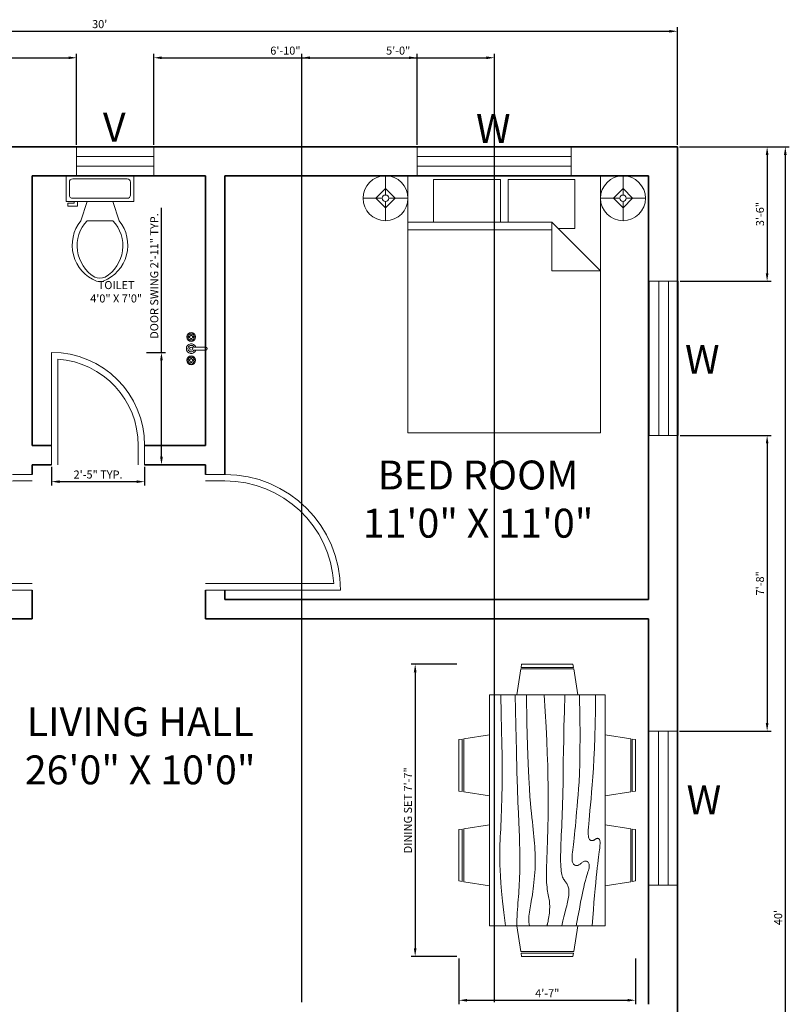
# Model space of a CAD drawing. Units: inches. Extents: x 1025 to 3479, y 1594 to 2212.
# Tile 3 of 9: x 1954 to 2194, y 1843 to 2150. Entities that reach past the tile are written whole.
import ezdxf

# ---------------------------------------------------------------- set-up
doc = ezdxf.new("R2010")
doc.units = ezdxf.units.IN
for name, color, linetype, lineweight in [('A-ANNO-DIMS', 1, 'Continuous', 18), ('A-ANNO-TEXT', 7, 'Continuous', 18), ('A-AREA-IDEN', 4, 'Continuous', 18), ('A-DOOR', 4, 'Continuous', 18), ('A-FLOR-FIXT', 9, 'Continuous', 18), ('A-FURN', 8, 'Continuous', 13), ('A-GLAZ', 3, 'Continuous', 18), ('A-WALL', 7, 'Continuous', 35)]:
    doc.layers.add(name, color=color, linetype=linetype, lineweight=lineweight)
doc.styles.get("Standard").update_dxf_attribs({"font": 'arial.ttf'})
doc.dimstyles.new('ISO-25', dxfattribs={"dimtxt": 2.5, "dimasz": 2.5, "dimexe": 1.25, "dimexo": 0.625, "dimtad": 1, "dimdec": 0, "dimlunit": 3, "dimtxsty": 'Standard', "dimcen": 2.5, "dimadec": 0, "dimazin": 0, "dimtfac": 1, "dimtdec": 0, "dimtmove": 0, "dimatfit": 3, "dimfxl": 1, "dimarcsym": 0})

# ---------------------------------------------------------------- blocks, each defined once
blk = doc.blocks.new('*D1')
at = {"layer": 'A-ANNO-DIMS', "color": 0, "lineweight": -2, "transparency": 16777216}
for p, q in [((1799.1, 2111.11), (1799.1, 2147.74)), ((1801.6, 2146.49), (2156.6, 2146.49)), ((2159.1, 2111.11), (2159.1, 2147.74))]:
    blk.add_line(p, q, dxfattribs=at)
at = {"layer": 'A-ANNO-DIMS', "color": 0, "transparency": 16777216}
for points in [[(1801.6, 2146.9), (1801.6, 2146.07), (1799.1, 2146.49)], [(2156.6, 2146.9), (2156.6, 2146.07), (2159.1, 2146.49)]]:
    blk.add_solid(points, dxfattribs=at)
at = {"layer": 'Defpoints', "color": 0, "transparency": 16777216}
for p in [(2159.1, 2146.49), (1799.1, 2110.49), (2159.1, 2110.49)]:
    blk.add_point(p, dxfattribs=at)
at = {"layer": 'A-ANNO-DIMS', "color": 0, "transparency": 16777216, "insert": (1979.1, 2148.39), "char_height": 2.5, "attachment_point": 5}
blk.add_mtext("30'", dxfattribs=at)
blk = doc.blocks.new('*D4')
at = {"layer": 'A-ANNO-DIMS', "color": 0, "lineweight": -2, "transparency": 16777216}
for p, q in [((2159.72, 2110.49), (2193.95, 2110.49)), ((2192.7, 2107.99), (2192.7, 1632.99)), ((2159.72, 1630.49), (2193.95, 1630.49))]:
    blk.add_line(p, q, dxfattribs=at)
at = {"layer": 'A-ANNO-DIMS', "color": 0, "transparency": 16777216}
for points in [[(2192.28, 2107.99), (2193.12, 2107.99), (2192.7, 2110.49)], [(2192.28, 1632.99), (2193.12, 1632.99), (2192.7, 1630.49)]]:
    blk.add_solid(points, dxfattribs=at)
at = {"layer": 'Defpoints', "color": 0, "transparency": 16777216}
for p in [(2159.1, 2110.49), (2159.1, 1630.49), (2192.7, 1630.49)]:
    blk.add_point(p, dxfattribs=at)
at = {"layer": 'A-ANNO-DIMS', "color": 0, "transparency": 16777216, "insert": (2190.8, 1870.49), "char_height": 2.5, "attachment_point": 5, "rotation": 90}
blk.add_mtext("40'", dxfattribs=at)
blk = doc.blocks.new('Dining Set - 36 x 72 in.')
for p, q in [((-22.2343, 26.00059), (-23.4847, 17.99762)), ((-22.2304, 26), (-5.7608, 26)), ((-22, 27.5), (-22.1562, 26.50042)), ((-5.8416, 26.5), (-22.1534, 26.5)), ((-22, 27.5), (-6, 27.5)), ((-5.8437, 26.49966), (-6, 27.5)), ((-4.5152, 17.99762), (-5.7655, 25.99926)), ((5.7657, 26.00059), (4.5153, 17.99762)), ((5.7696, 26), (22.2392, 26)), ((6, 27.5), (5.8438, 26.50042)), ((22.1584, 26.5), (5.8466, 26.5)), ((6, 27.5), (22, 27.5)), ((22.1563, 26.49966), (22, 27.5)), ((23.4848, 17.99762), (22.2345, 25.99926)), ((36, 18), (-36, 18)), ((-36, 18), (-36, -18)), ((36, -18), (36, 18)), ((-44.0006, 8.23428), (-35.9976, 9.48474)), ((44.0006, 8.23428), (35.9976, 9.48474)), ((-45.5, 8), (-44.5004, 8.15617)), ((-45.5, 8), (-45.5, -8)), ((-44.5, -8.15843), (-44.5, 8.15338)), ((-44, 8.23041), (-44, -8.23915)), ((44, 8.23041), (44, -8.23915)), ((44.5, -8.15843), (44.5, 8.15338)), ((45.5, 8), (44.5005, 8.15617)), ((45.5, 8), (45.5, -8)), ((-44.4997, -8.15631), (-45.5, -8)), ((-35.9976, -9.48476), (-43.9993, -8.2345)), ((35.9976, -9.48476), (43.9993, -8.2345)), ((44.4997, -8.15631), (45.5, -8)), ((-36, -18), (36, -18)), ((-22.2343, -26.0006), (-23.4847, -17.99762)), ((-4.5152, -17.99762), (-5.7655, -25.99928)), ((5.7657, -26.0006), (4.5153, -17.99762)), ((23.4848, -17.99762), (22.2345, -25.99928)), ((-22.2304, -26), (-5.7608, -26)), ((-22, -27.5), (-22.1562, -26.50044)), ((-5.8416, -26.5), (-22.1534, -26.5)), ((-22, -27.5), (-6, -27.5)), ((-5.8437, -26.49967), (-6, -27.5)), ((5.7696, -26), (22.2392, -26)), ((6, -27.5), (5.8438, -26.50044)), ((22.1584, -26.5), (5.8466, -26.5)), ((6, -27.5), (22, -27.5)), ((22.1563, -26.49967), (22, -27.5))]:
    blk.add_line(p, q)
for points in [[(-36, 15), (-31.1772, 14.97754), (-26.8079, 14.91406), (-22.8538, 14.81543), (-19.276, 14.6875), (-16.0362, 14.53613), (-13.0957, 14.36718), (-10.4159, 14.18652), (-7.9583, 14), (-5.6904, 13.81315), (-3.6035, 13.63021), (-1.6954, 13.45508), (0.0365, 13.29166), (1.5945, 13.14388), (2.9811, 13.01562), (4.1988, 12.9108), (5.25, 12.83333), (6.1393, 12.78613), (6.8802, 12.76823), (7.4883, 12.77767), (7.9792, 12.8125), (8.3685, 12.87077), (8.6719, 12.95052), (8.9049, 13.0498), (9.0833, 13.16666), (9.2205, 13.29899), (9.3216, 13.44401), (9.3895, 13.59879), (9.4271, 13.76041), (9.4373, 13.92594), (9.4232, 14.09245), (9.3875, 14.257), (9.3333, 14.41666), (9.2638, 14.56917), (9.1836, 14.71484), (9.0975, 14.85465), (9.0104, 14.98958), (8.9272, 15.1206), (8.8529, 15.2487), (8.7922, 15.37483), (8.75, 15.5), (8.7305, 15.62467), (8.7344, 15.74739), (8.7617, 15.86621), (8.8125, 15.97916), (8.8867, 16.08431), (8.9844, 16.17968), (9.1055, 16.26334), (9.25, 16.33333), (9.4189, 16.38802), (9.6172, 16.42708), (9.8506, 16.45052), (10.125, 16.45833), (10.4463, 16.45052), (10.8203, 16.42708), (11.2529, 16.38802), (11.75, 16.33333), (12.3184, 16.26318), (12.9694, 16.17838), (13.7151, 16.07991), (14.5677, 15.96875), (15.5395, 15.84586), (16.6426, 15.71224), (17.8893, 15.56884), (19.2917, 15.41666), (20.859, 15.25667), (22.5879, 15.08984), (24.4721, 14.91715), (26.5052, 14.73958), (28.6809, 14.5581), (30.9929, 14.3737), (33.4347, 14.18733), (36, 14)], [(-36, 10), (-28.9766, 10.14274), (-23.1725, 10.20442), (-18.4241, 10.19775), (-14.5677, 10.13541), (-11.4399, 10.03011), (-8.877, 9.89453), (-6.7154, 9.74137), (-4.7917, 9.58333), (-2.9698, 9.43082), (-1.2246, 9.28515), (0.4415, 9.14534), (2.026, 9.01041), (3.5266, 8.87939), (4.9408, 8.7513), (6.266, 8.62516), (7.5, 8.5), (8.6411, 8.37549), (9.6914, 8.2539), (10.6538, 8.13818), (11.5312, 8.03125), (12.3267, 7.93603), (13.043, 7.85547), (13.6831, 7.79248), (14.25, 7.75), (14.7471, 7.7303), (15.1797, 7.73307), (15.5537, 7.75732), (15.875, 7.80208), (16.1494, 7.86637), (16.3828, 7.94922), (16.5811, 8.04964), (16.75, 8.16666), (16.8944, 8.29915), (17.0143, 8.44531), (17.1089, 8.60319), (17.1771, 8.77083), (17.218, 8.94629), (17.2305, 9.1276), (17.2137, 9.31282), (17.1667, 9.5), (17.0895, 9.6875), (16.987, 9.875), (16.8649, 10.0625), (16.7292, 10.25), (16.5856, 10.4375), (16.4401, 10.625), (16.2985, 10.8125), (16.1667, 11), (16.05, 11.18733), (15.9518, 11.3737), (15.8752, 11.5581), (15.8229, 11.73958), (15.798, 11.91715), (15.8034, 12.08984), (15.842, 12.25667), (15.9167, 12.41666), (16.0295, 12.56836), (16.1784, 12.70833), (16.3605, 12.83268), (16.5729, 12.9375), (16.8127, 13.01888), (17.0768, 13.07291), (17.3625, 13.0957), (17.6667, 13.08333), (17.9894, 13.03312), (18.3418, 12.94726), (18.7382, 12.82918), (19.1927, 12.68229), (19.7195, 12.51001), (20.3327, 12.31575), (21.0465, 12.10294), (21.875, 11.875), (22.8357, 11.63354), (23.959, 11.37304), (25.2786, 11.08618), (26.8282, 10.76562), (28.6414, 10.40405), (30.752, 9.99414), (33.1936, 9.52856), (36, 9)], [(-36, 5.5), (-30.7157, 5.3348), (-26.069, 5.20963), (-21.9946, 5.11767), (-18.4271, 5.05208), (-15.3009, 5.00602), (-12.5508, 4.97265), (-10.1112, 4.94515), (-7.9167, 4.91666), (-5.909, 4.88167), (-4.0586, 4.83984), (-2.3429, 4.79215), (-0.7396, 4.73958), (0.7739, 4.6831), (2.22, 4.6237), (3.6213, 4.56233), (5, 4.5), (6.373, 4.43782), (7.7344, 4.3776), (9.0723, 4.32129), (10.375, 4.27083), (11.6309, 4.22819), (12.8281, 4.19531), (13.9551, 4.17415), (15, 4.16666), (15.954, 4.17448), (16.819, 4.19791), (17.6001, 4.23698), (18.3021, 4.29166), (18.9299, 4.36198), (19.4883, 4.44791), (19.9823, 4.54948), (20.4167, 4.66666), (20.7969, 4.79899), (21.1302, 4.94401), (21.4245, 5.09879), (21.6875, 5.26041), (21.9271, 5.42594), (22.1511, 5.59245), (22.3672, 5.757), (22.5834, 5.91666), (22.8065, 6.06868), (23.0404, 6.21093), (23.2879, 6.34147), (23.5521, 6.45833), (23.8358, 6.55957), (24.142, 6.64323), (24.4735, 6.70735), (24.8334, 6.75), (25.2235, 6.76969), (25.642, 6.76692), (26.0858, 6.74267), (26.5521, 6.69791), (27.0379, 6.63362), (27.5404, 6.55078), (28.0565, 6.45036), (28.5834, 6.33333), (29.1242, 6.19987), (29.7071, 6.04687), (30.3661, 5.87044), (31.1354, 5.66666), (32.0493, 5.43164), (33.142, 5.16146), (34.4475, 4.85221), (36, 4.5)], [(-36, -1), (-30.7915, -0.6591), (-26.0195, -0.38216), (-21.6519, -0.16284), (-17.6563, 0.00521), (-14.0005, 0.12833), (-10.6523, 0.21289), (-7.5796, 0.26522), (-4.75, 0.29166), (-2.134, 0.29793), (0.2878, 0.28711), (2.5317, 0.26163), (4.6146, 0.22396), (6.5529, 0.17651), (8.3633, 0.12174), (10.0623, 0.06209), (11.6667, 0), (13.1899, -0.06201), (14.6341, -0.1211), (15.9982, -0.17432), (17.2813, -0.21875), (18.4823, -0.25147), (19.6003, -0.26953), (20.6343, -0.27002), (21.5834, -0.25), (22.4481, -0.20768), (23.2357, -0.14584), (23.9549, -0.06836), (24.6146, 0.02083), (25.2235, 0.11784), (25.7904, 0.21875), (26.3241, 0.31966), (26.8334, 0.41666), (27.3265, 0.50618), (27.8099, 0.58593), (28.2894, 0.65397), (28.7709, 0.70833), (29.2601, 0.74707), (29.763, 0.76823), (30.2855, 0.76985), (30.8334, 0.75), (31.4088, 0.70784), (31.9994, 0.64713), (32.589, 0.57275), (33.1615, 0.48958), (33.7008, 0.4025), (34.1908, 0.3164), (34.6153, 0.23616), (34.9584, 0.16666), (35.2099, 0.11165), (35.3848, 0.07031), (35.504, 0.04069), (35.5886, 0.02083), (35.6594, 0.00879), (35.7377, 0.0026), (35.8442, 0.00032), (36, 0)], [(-36, -6.5), (-27.1843, -6.31267), (-20.084, -6.1263), (-14.469, -5.9419), (-10.1094, -5.76042), (-6.7752, -5.58285), (-4.2363, -5.41016), (-2.2629, -5.24333), (-0.625, -5.08334), (0.8708, -4.93099), (2.2715, -4.78646), (3.5872, -4.64974), (4.8281, -4.52084), (6.0046, -4.39974), (7.127, -4.28646), (8.2053, -4.18099), (9.25, -4.08334), (10.2705, -3.99382), (11.2734, -3.91407), (12.2647, -3.84603), (13.25, -3.79167), (14.2354, -3.75293), (15.2266, -3.73177), (16.2295, -3.73015), (17.25, -3.75), (18.2912, -3.79248), (19.3451, -3.85547), (20.4009, -3.93604), (21.4479, -4.03125), (22.4754, -4.13819), (23.4727, -4.25391), (24.4289, -4.37549), (25.3334, -4.5), (26.1785, -4.62492), (26.9694, -4.74935), (27.7145, -4.87281), (28.4219, -4.99479), (29.1, -5.11483), (29.7572, -5.23242), (30.4016, -5.34709), (31.0417, -5.45834), (31.6837, -5.56437), (32.3262, -5.65821), (32.9658, -5.73153), (33.599, -5.77604), (34.2224, -5.78345), (34.8327, -5.74545), (35.4264, -5.65373), (36, -5.5)], [(-36, -10), (-26.4022, -9.81299), (-18.4675, -9.62891), (-11.9839, -9.45069), (-6.7396, -9.28125), (-2.5226, -9.12354), (0.8789, -8.98047), (3.6769, -8.85498), (6.0833, -8.75), (8.2767, -8.66765), (10.3021, -8.60677), (12.1712, -8.56543), (13.8958, -8.54167), (15.4876, -8.53353), (16.9583, -8.53907), (18.3197, -8.55632), (19.5834, -8.58334), (20.7616, -8.61841), (21.8685, -8.66081), (22.9188, -8.71004), (23.9271, -8.76563), (24.9081, -8.82707), (25.8763, -8.89388), (26.8465, -8.96558), (27.8334, -9.04167), (28.8474, -9.12118), (29.8828, -9.20117), (30.93, -9.27824), (31.9792, -9.34896), (33.0205, -9.40991), (34.0443, -9.45768), (35.0407, -9.48885), (36, -9.5)], [(-36, -14.5), (-30.0881, -14.33513), (-25.0332, -14.21224), (-20.7312, -14.12647), (-17.0781, -14.07292), (-13.97, -14.04671), (-11.3027, -14.04297), (-8.9724, -14.05681), (-6.875, -14.08334), (-4.9224, -14.11833), (-3.0905, -14.16016), (-1.3709, -14.20785), (0.2448, -14.26042), (1.7647, -14.3169), (3.1973, -14.3763), (4.5507, -14.43767), (5.8333, -14.5), (7.0554, -14.5621), (8.235, -14.62175), (9.3922, -14.67652), (10.5469, -14.72396), (11.7192, -14.76164), (12.929, -14.78711), (14.1965, -14.79794), (15.5417, -14.79167), (16.9933, -14.76424), (18.6152, -14.70508), (20.4804, -14.60197), (22.6615, -14.44271), (25.2312, -14.21509), (28.2624, -13.9069), (31.8277, -13.50594), (36, -13)]]:
    blk.add_lwpolyline(points)
blk = doc.blocks.new('Bed - Queen')
for p, q in [((0, -80.00003), (0, 0)), ((0, 0), (59.99999, 0)), ((59.99999, 0), (59.99999, -80.00003)), ((7.99999, -1.2), (28.79998, -1.2)), ((7.99999, -14.4), (7.99999, -1.2)), ((28.79998, -1.2), (28.79998, -14.4)), ((31.19999, -1.2), (51.99999, -1.2)), ((31.19999, -14.4), (31.19999, -1.2)), ((51.99999, -1.2), (51.99999, -16.4)), ((0, -14.4), (44.8, -14.4)), ((59.99999, -29.6), (44.8, -14.4)), ((44.8, -14.4), (44.8, -29.6)), ((44.8, -16.8), (0, -16.8)), ((51.99999, -16.4), (46.79936, -16.4)), ((44.8, -29.6), (59.99999, -29.6)), ((59.99999, -80.00003), (0, -80.00003))]:
    blk.add_line(p, q)
blk = doc.blocks.new('Lamp - Table')
for p, q in [((0, 7), (0, 1)), ((-1, 0), (-7, 0)), ((0, 3), (-3, 0)), ((-3, 0), (0, -3)), ((3, 0), (0, 3)), ((0, -3), (3, 0)), ((1, 0), (7, 0)), ((0, -1), (0, -7))]:
    blk.add_line(p, q)
for radius in [7, 1]:
    blk.add_circle((0, 0), radius)
blk = doc.blocks.new('Toilet - top')
for p, q in [((9.5, -6), (9.5, -2)), ((-10, -8.5), (-8, -8.5)), ((-10, -9.5), (-10, -8.5)), ((-8, -8.5), (-8, -8)), ((-7, -8), (-7, -9.5)), ((-4, -8), (-6, -14)), ((4, -8), (6, -14)), ((-7, -9.5), (-10, -9.5)), ((4, -14), (-4, -14))]:
    blk.add_line(p, q)
blk.add_lwpolyline([(10.5, -8), (10.5, 0), (-10.5, 0), (-10.5, -8)], close=True)
for points in [[(-9.5, -2), (-9.5, -6)], [(8.5, -1), (-8.5, -1)], [(-8.5, -7), (8.5, -7)]]:
    blk.add_lwpolyline(points)
for centre, radius, start, end in [((-8.62, -1.88), 0.884, 81.8699, 188.1301), ((8.62, -1.88), 0.884, 351.8699, 98.1301), ((-8.62, -6.12), 0.884, 171.8699, 278.1301), ((8.62, -6.12), 0.884, 261.8699, 8.1301), ((3.52, -21.58), 12.17, 141.4691, 247.9714), ((4.2, -21.82), 11.33, 136.3677, 238.9468), ((-3.52, -21.58), 12.17, 292.0284, 38.5307), ((-4.2, -21.82), 11.33, 301.053, 43.6321), ((0, -27.88), 4, 245.7318, 294.2682), ((0, -29), 4, 254.8605, 285.1395)]:
    blk.add_arc(centre, radius, start, end)
blk = doc.blocks.new('Faucet - Bathroom top')
for p, q in [((-4.107, 0.125), (-4.375, 0.125)), ((-3.75, 0.4788), (-3.75, 0.75)), ((-3.5, 0.482), (-3.5, 0.75)), ((-3.1461, 0.125), (-2.875, 0.125)), ((3.143, 0.125), (2.875, 0.125)), ((3.5, 0.4788), (3.5, 0.75)), ((3.75, 0.482), (3.75, 0.75)), ((4.1039, 0.125), (4.375, 0.125)), ((-4.1039, -0.125), (-4.375, -0.125)), ((-3.75, -0.4821), (-3.75, -0.75)), ((-3.5, -0.4789), (-3.5, -0.75)), ((-3.143, -0.125), (-2.875, -0.125)), ((-0.5, -0.8639), (-0.5, -4.5)), ((0.5, -4.5), (0.5, -0.8631)), ((3.1461, -0.125), (2.875, -0.125)), ((3.5, -0.4821), (3.5, -0.75)), ((3.75, -0.4789), (3.75, -0.75)), ((4.107, -0.125), (4.375, -0.125))]:
    blk.add_line(p, q)
for centre, radius in [((-3.625, 0), 1.375), ((-4.625, 0), 0.2795), ((-3.625, 0), 0.5), ((-3.625, 1), 0.2795), ((-2.625, 0), 0.2795), ((0, 0), 0.5), ((3.625, 0), 1.375), ((2.625, 0), 0.2795), ((3.625, 0), 0.5), ((3.625, 1), 0.2795), ((4.625, 0), 0.2795), ((-3.625, -1), 0.2795), ((3.625, -1), 0.2795)]:
    blk.add_circle(centre, radius)
for centre, radius, start, end in [((-3.625, 0), 1, 105.2407, 164.2093), ((-3.625, 0), 1, 16.44125, 74.07887), ((0, 0), 1.5, 289.6514, 250.3603), ((0, 0), 1, 300.3431, 239.7554), ((3.625, 0), 1, 106.12, 164.0884), ((3.625, 0), 1, 16.23422, 73.90469), ((-3.625, 0), 1, 196.2342, 253.9047), ((-3.625, 0), 1, 286.12, 344.0884), ((3.625, 0), 1, 196.4413, 254.0789), ((3.625, 0), 1, 285.2407, 344.2093), ((0, -4.5), 0.5, 180, 0)]:
    blk.add_arc(centre, radius, start, end)
blk = doc.blocks.new('WIN-48IN')
for p, q in [((0, 48), (0, 0)), ((9, 48), (0, 48)), ((3, 48), (3, 0)), ((6, 0), (6, 48)), ((9, 0), (9, 48)), ((0, 0), (9, 0))]:
    blk.add_line(p, q)
blk = doc.blocks.new('VENT-24IN')
for p, q in [((24, 9), (0, 9)), ((0, 9), (0, 0)), ((24, 0), (24, 9)), ((24, 6), (0, 6)), ((0, 3), (24, 3)), ((0, 0), (24, 0))]:
    blk.add_line(p, q)
blk = doc.blocks.new('DOOR-SWING-36IN')
for p, q in [((0, 36), (6, 36)), ((0, 34), (6, 34)), ((0, 2), (6, 2)), ((6, 0), (0, 0)), ((6, 2), (39.94, 2)), ((6, 0), (42, 0))]:
    blk.add_line(p, q)
for radius, start in [(36, 0), (34, 3.3723)]:
    blk.add_arc((6, 0), radius, start, 90)
blk = doc.blocks.new('DOOR-SWING-29IN')
for p, q in [((0, 6), (0, 35)), ((2, 6), (2, 32.93)), ((0, 6), (0, 0)), ((2, 6), (2, 0)), ((27, 0), (27, 6)), ((29, 0), (29, 6))]:
    blk.add_line(p, q)
for radius, end in [(29, 90), (27, 85.752)]:
    blk.add_arc((0, 6), radius, 0, end)
blk = doc.blocks.new('*D34')
at = {"layer": 'A-ANNO-DIMS', "color": 0, "lineweight": -2, "transparency": 16777216}
for p, q in [((1998.35, 2046.49), (1998.35, 2091.55)), ((1993.72, 2046.49), (1999.6, 2046.49)), ((1998.35, 2013.99), (1998.35, 2043.99)), ((1993.72, 2011.49), (1999.6, 2011.49))]:
    blk.add_line(p, q, dxfattribs=at)
at = {"layer": 'A-ANNO-DIMS', "color": 0, "transparency": 16777216}
for points in [[(1997.93, 2043.99), (1998.77, 2043.99), (1998.35, 2046.49)], [(1997.93, 2013.99), (1998.77, 2013.99), (1998.35, 2011.49)]]:
    blk.add_solid(points, dxfattribs=at)
at = {"layer": 'Defpoints', "color": 0, "transparency": 16777216}
for p in [(1993.1, 2046.49), (1998.35, 2046.49), (1993.1, 2011.49)]:
    blk.add_point(p, dxfattribs=at)
at = {"layer": 'A-ANNO-DIMS', "color": 0, "transparency": 16777216, "insert": (1996.43, 2070.27), "char_height": 2.5, "attachment_point": 5, "rotation": 90}
blk.add_mtext('DOOR SWING 2\'-11" TYP.', dxfattribs=at)
blk = doc.blocks.new('*D35')
at = {"layer": 'A-ANNO-DIMS', "color": 0, "lineweight": -2, "transparency": 16777216}
for p, q in [((1964.1, 2010.86), (1964.1, 2004.99)), ((1993.1, 2010.86), (1993.1, 2004.99)), ((1966.6, 2006.24), (1990.6, 2006.24))]:
    blk.add_line(p, q, dxfattribs=at)
at = {"layer": 'A-ANNO-DIMS', "color": 0, "transparency": 16777216}
for points in [[(1966.6, 2006.65), (1966.6, 2005.82), (1964.1, 2006.24)], [(1990.6, 2006.65), (1990.6, 2005.82), (1993.1, 2006.24)]]:
    blk.add_solid(points, dxfattribs=at)
at = {"layer": 'Defpoints', "color": 0, "transparency": 16777216}
for p in [(1964.1, 2011.49), (1993.1, 2011.49), (1993.1, 2006.24)]:
    blk.add_point(p, dxfattribs=at)
at = {"layer": 'A-ANNO-DIMS', "color": 0, "transparency": 16777216, "insert": (1978.6, 2008.14), "char_height": 2.5, "attachment_point": 5}
blk.add_mtext('2\'-5" TYP.', dxfattribs=at)
blk = doc.blocks.new('*D44')
at = {"layer": 'A-ANNO-DIMS', "color": 0, "lineweight": -2, "transparency": 16777216}
for p, q in [((2090.41, 1949.4), (2076.14, 1949.4)), ((2077.39, 1946.9), (2077.39, 1860.9)), ((2090.41, 1858.4), (2076.14, 1858.4))]:
    blk.add_line(p, q, dxfattribs=at)
at = {"layer": 'A-ANNO-DIMS', "color": 0, "transparency": 16777216}
for points in [[(2076.97, 1946.9), (2077.81, 1946.9), (2077.39, 1949.4)], [(2076.97, 1860.9), (2077.81, 1860.9), (2077.39, 1858.4)]]:
    blk.add_solid(points, dxfattribs=at)
at = {"layer": 'Defpoints', "color": 0, "transparency": 16777216}
for p in [(2091.04, 1949.4), (2077.39, 1858.4), (2091.04, 1858.4)]:
    blk.add_point(p, dxfattribs=at)
at = {"layer": 'A-ANNO-DIMS', "color": 0, "transparency": 16777216, "insert": (2075.47, 1903.9), "char_height": 2.5, "attachment_point": 5, "rotation": 90}
blk.add_mtext('DINING SET 7\'-7"', dxfattribs=at)
blk = doc.blocks.new('*D45')
at = {"layer": 'A-ANNO-DIMS', "color": 0, "lineweight": -2, "transparency": 16777216}
for p, q in [((2091.04, 1857.77), (2091.04, 1843.5)), ((2146.04, 1857.77), (2146.04, 1843.5)), ((2093.54, 1844.75), (2143.54, 1844.75))]:
    blk.add_line(p, q, dxfattribs=at)
at = {"layer": 'A-ANNO-DIMS', "color": 0, "transparency": 16777216}
for points in [[(2093.54, 1845.16), (2093.54, 1844.33), (2091.04, 1844.75)], [(2143.54, 1845.16), (2143.54, 1844.33), (2146.04, 1844.75)]]:
    blk.add_solid(points, dxfattribs=at)
at = {"layer": 'Defpoints', "color": 0, "transparency": 16777216}
for p in [(2091.04, 1858.4), (2146.04, 1858.4), (2146.04, 1844.75)]:
    blk.add_point(p, dxfattribs=at)
at = {"layer": 'A-ANNO-DIMS', "color": 0, "transparency": 16777216, "insert": (2118.54, 1846.62), "char_height": 2.5, "attachment_point": 5}
blk.add_mtext('4\'-7"', dxfattribs=at)
blk = doc.blocks.new('*D50')
at = {"layer": 'A-ANNO-DIMS', "color": 0, "lineweight": -2, "transparency": 16777216}
for p, q in [((1876.48, 2111.11), (1876.48, 2139.49)), ((1878.98, 2138.24), (1969.43, 2138.24)), ((1971.93, 2111.11), (1971.93, 2139.49))]:
    blk.add_line(p, q, dxfattribs=at)
at = {"layer": 'A-ANNO-DIMS', "color": 0, "transparency": 16777216}
for points in [[(1878.98, 2138.65), (1878.98, 2137.82), (1876.48, 2138.24)], [(1969.43, 2138.65), (1969.43, 2137.82), (1971.93, 2138.24)]]:
    blk.add_solid(points, dxfattribs=at)
at = {"layer": 'Defpoints', "color": 0, "transparency": 16777216}
for p in [(1971.93, 2138.24), (1876.48, 2110.49), (1971.93, 2110.49)]:
    blk.add_point(p, dxfattribs=at)
at = {"layer": 'A-ANNO-DIMS', "color": 0, "transparency": 16777216, "insert": (1924.21, 2140.15), "char_height": 2.5, "attachment_point": 5}
blk.add_mtext('7\'-11 1/2"', dxfattribs=at)
blk = doc.blocks.new('*D51')
at = {"layer": 'A-ANNO-DIMS', "color": 0, "lineweight": -2, "transparency": 16777216}
for p, q in [((1995.93, 2111.11), (1995.93, 2139.49)), ((1998.43, 2138.24), (2075.48, 2138.24)), ((2077.98, 2111.11), (2077.98, 2139.49))]:
    blk.add_line(p, q, dxfattribs=at)
at = {"layer": 'A-ANNO-DIMS', "color": 0, "transparency": 16777216}
for points in [[(1998.43, 2138.65), (1998.43, 2137.82), (1995.93, 2138.24)], [(2075.48, 2138.65), (2075.48, 2137.82), (2077.98, 2138.24)]]:
    blk.add_solid(points, dxfattribs=at)
at = {"layer": 'Defpoints', "color": 0, "transparency": 16777216}
for p in [(2077.98, 2138.24), (1995.93, 2110.49), (2077.98, 2110.49)]:
    blk.add_point(p, dxfattribs=at)
at = {"layer": 'A-ANNO-DIMS', "color": 0, "transparency": 16777216, "insert": (2036.96, 2140.14), "char_height": 2.5, "attachment_point": 5}
blk.add_mtext('6\'-10"', dxfattribs=at)
blk = doc.blocks.new('*D69')
at = {"layer": 'A-ANNO-DIMS', "color": 0, "lineweight": -2, "transparency": 16777216}
for p, q in [((2159.72, 2110.49), (2188.29, 2110.49)), ((2187.04, 2107.99), (2187.04, 2071.13)), ((2159.91, 2068.63), (2188.29, 2068.63))]:
    blk.add_line(p, q, dxfattribs=at)
at = {"layer": 'A-ANNO-DIMS', "color": 0, "transparency": 16777216}
for points in [[(2186.62, 2107.99), (2187.46, 2107.99), (2187.04, 2110.49)], [(2186.62, 2071.13), (2187.46, 2071.13), (2187.04, 2068.63)]]:
    blk.add_solid(points, dxfattribs=at)
at = {"layer": 'Defpoints', "color": 0, "transparency": 16777216}
for p in [(2159.1, 2110.49), (2159.29, 2068.63), (2187.04, 2068.63)]:
    blk.add_point(p, dxfattribs=at)
at = {"layer": 'A-ANNO-DIMS', "color": 0, "transparency": 16777216, "insert": (2185.14, 2089.56), "char_height": 2.5, "attachment_point": 5, "rotation": 90}
blk.add_mtext('3\'-6"', dxfattribs=at)
blk = doc.blocks.new('*D70')
at = {"layer": 'A-ANNO-DIMS', "color": 0, "lineweight": -2, "transparency": 16777216}
for p, q in [((2159.91, 2020.63), (2188.29, 2020.63)), ((2187.04, 2018.13), (2187.04, 1931.05)), ((2159.78, 1928.55), (2188.29, 1928.55))]:
    blk.add_line(p, q, dxfattribs=at)
at = {"layer": 'A-ANNO-DIMS', "color": 0, "transparency": 16777216}
for points in [[(2186.62, 2018.13), (2187.46, 2018.13), (2187.04, 2020.63)], [(2186.62, 1931.05), (2187.46, 1931.05), (2187.04, 1928.55)]]:
    blk.add_solid(points, dxfattribs=at)
at = {"layer": 'Defpoints', "color": 0, "transparency": 16777216}
for p in [(2159.29, 2020.63), (2159.16, 1928.55), (2187.04, 1928.55)]:
    blk.add_point(p, dxfattribs=at)
at = {"layer": 'A-ANNO-DIMS', "color": 0, "transparency": 16777216, "insert": (2185.14, 1974.59), "char_height": 2.5, "attachment_point": 5, "rotation": 90}
blk.add_mtext('7\'-8"', dxfattribs=at)
blk = doc.blocks.new('*D84')
at = {"layer": 'A-ANNO-DIMS', "color": 0, "lineweight": -2, "transparency": 16777216}
for p, q in [((2042.1, 1844.11), (2042.1, 2139.49)), ((2044.6, 2138.24), (2099.6, 2138.24)), ((2102.1, 1844.11), (2102.1, 2139.49))]:
    blk.add_line(p, q, dxfattribs=at)
at = {"layer": 'A-ANNO-DIMS', "color": 0, "transparency": 16777216}
for points in [[(2044.6, 2138.65), (2044.6, 2137.82), (2042.1, 2138.24)], [(2099.6, 2138.65), (2099.6, 2137.82), (2102.1, 2138.24)]]:
    blk.add_solid(points, dxfattribs=at)
at = {"layer": 'Defpoints', "color": 0, "transparency": 16777216}
for p in [(2102.1, 2138.24), (2042.1, 1843.49), (2102.1, 1843.49)]:
    blk.add_point(p, dxfattribs=at)
at = {"layer": 'A-ANNO-DIMS', "color": 0, "transparency": 16777216, "insert": (2072.1, 2140.14), "char_height": 2.5, "attachment_point": 5}
blk.add_mtext('5\'-0"', dxfattribs=at)

msp = doc.modelspace()

# ---------------------------------------------------------------- linework, layer by layer
at = {"layer": 'A-DOOR'}
for p, q in [((1958.1, 1972.49), (1952.1, 1972.49)), ((2012.1, 1972.49), (2018.1, 1972.49))]:
    msp.add_line(p, q, dxfattribs=at)
at = {"layer": 'A-WALL'}
for p, q in [((1799.1, 2110.49), (2159.1, 2110.49)), ((2159.1, 2110.49), (2159.1, 1630.49)), ((1958.1, 2101.49), (2012.1, 2101.49)), ((1958.1, 2017.49), (1958.1, 2101.49)), ((1958.1, 2017.49), (1958.1, 2101.49)), ((2012.1, 2101.49), (2012.1, 2017.49)), ((2018.1, 2101.49), (2018.1, 2008.49)), ((2018.1, 2101.49), (2150.1, 2101.49)), ((2150.1, 2101.49), (2150.1, 1969.49)), ((1958.1, 2017.49), (1964.1, 2017.49)), ((1958.1, 2017.49), (1964.1, 2017.49)), ((1993.1, 2017.49), (2012.1, 2017.49)), ((1958.1, 2011.49), (1964.1, 2011.49)), ((1958.1, 2011.49), (1958.1, 2011.49)), ((1958.1, 2011.49), (1958.1, 2008.49)), ((1958.1, 2008.49), (1958.1, 2011.49)), ((1958.1, 2008.49), (1958.1, 2011.49)), ((1993.1, 2011.49), (2012.1, 2011.49)), ((2012.1, 2011.49), (2012.1, 2008.49)), ((2012.1, 2011.49), (2012.1, 2008.49)), ((1958.1, 1963.49), (1958.1, 1972.49)), ((1958.1, 1963.49), (1958.1, 1972.49)), ((2012.1, 1972.49), (2012.1, 1963.49)), ((2018.1, 1972.49), (2018.1, 1969.49)), ((2018.1, 1969.49), (2150.1, 1969.49)), ((1808.1, 1963.49), (1958.1, 1963.49)), ((2012.1, 1963.49), (2150.1, 1963.49)), ((2150.1, 1963.49), (2150.1, 1843.49))]:
    msp.add_line(p, q, dxfattribs=at)

# ---------------------------------------------------------------- block references
at = {"layer": 'A-DOOR'}
for name, p in [('DOOR-SWING-29IN', (1964.1, 2011.49)), ('DOOR-SWING-36IN', (2012.1, 1972.49))]:
    msp.add_blockref(name, p, dxfattribs=at)
at = {"layer": 'A-DOOR', "extrusion": (0, 0, -1), "zscale": -1}
msp.add_blockref('DOOR-SWING-36IN', (-1958.1, 1972.49), dxfattribs=at)
at = {"layer": 'A-FLOR-FIXT'}
msp.add_blockref('Toilet - top', (1979.19, 2101.49), dxfattribs=at)
at = {"layer": 'A-FLOR-FIXT', "rotation": 90}
msp.add_blockref('Faucet - Bathroom top', (2007.6, 2047.66), dxfattribs=at)
at = {"layer": 'A-FURN'}
for name, p in [('Lamp - Table', (2068.14, 2094.49)), ('Bed - Queen', (2075.14, 2101.49)), ('Lamp - Table', (2142.14, 2094.49))]:
    msp.add_blockref(name, p, dxfattribs=at)
at = {"layer": 'A-FURN', "rotation": 270}
msp.add_blockref('Dining Set - 36 x 72 in.', (2118.54, 1903.9), dxfattribs=at)
at = {"layer": 'A-GLAZ'}
for name, p in [('VENT-24IN', (1971.93, 2101.49)), ('WIN-48IN', (2150.29, 2020.63)), ('WIN-48IN', (2150.16, 1880.55))]:
    msp.add_blockref(name, p, dxfattribs=at)
at = {"layer": 'A-GLAZ', "rotation": 269.9999999999989}
msp.add_blockref('WIN-48IN', (2077.98, 2110.49), dxfattribs=at)

# ---------------------------------------------------------------- texts
at = {"layer": 'A-ANNO-TEXT', "char_height": 9, "attachment_point": 1}
for s, width, insert in [('\\pxqc;{V}', 7.8272, (1979.73, 2121.13)), ('\\pxqc;W', 15.8719, (2093.79, 2120.73)), ('\\pxqc;W', 15.8719, (2158.9, 2048.84)), ('\\pxqc;W', 15.8719, (2159.41, 1911.64))]:
    msp.add_mtext_dynamic_manual_height_columns(s, width=width, gutter_width=12.5, heights=[0], dxfattribs=dict(at, insert=insert))
at = {"layer": 'A-AREA-IDEN', "attachment_point": 1}
for s, width, insert, char_height in [('\\pxqc;TOILET\\P4\'0" X 7\'0"', 47.6002, (1960.44, 2068.7), 2.5), ('\\pxqc;BED ROOM \\P11\'0" X 11\'0"', 93.2353, (2050.37, 2012.8), 9), ('\\pxqc;LIVING HALL\\P26\'0" X 10\'0"', 112.2145, (1935.6, 1935.99), 9)]:
    msp.add_mtext_dynamic_manual_height_columns(s, width=width, gutter_width=12.5, heights=[0], dxfattribs=dict(at, insert=insert, char_height=char_height))

# ---------------------------------------------------------------- dimensions: what is measured, and where the dimension line sits
at = {"layer": 'A-ANNO-DIMS'}
for base, p1, p2, override, picture, middle in [((2159.1, 2146.49), (1799.1, 2110.49), (2159.1, 2110.49), {"dimclrd": 0, "dimclre": 0, "dimclrt": 0}, '*D1', (1979.1, 2148.39)), ((1971.9348, 2138.2355), (1876.4813, 2110.4855), (1971.9348, 2110.4855), {"dimdec": 1, "dimlfac": 1, "dimrnd": 0, "dimzin": 1, "dimdsep": 46, "dimlunit": 4, "dimfrac": 2}, '*D50', (1924.208, 2140.1532)), ((2077.9791, 2138.2355), (1995.9348, 2110.4855), (2077.9791, 2110.4855), {"dimdec": 1, "dimlfac": 1, "dimrnd": 0, "dimzin": 1, "dimdsep": 46, "dimlunit": 4, "dimfrac": 2}, '*D51', (2036.9569, 2140.137)), ((2102.1, 2138.24), (2042.1, 1843.49), (2102.1, 1843.49), {"dimdec": 1, "dimlfac": 1, "dimrnd": 0, "dimzin": 1, "dimdsep": 46, "dimlunit": 4, "dimfrac": 2}, '*D84', (2072.1, 2140.14)), ((2146.04, 1844.75), (2091.04, 1858.4), (2146.04, 1858.4), {"dimdec": 1, "dimlfac": 1, "dimrnd": 0, "dimzin": 1, "dimdsep": 46, "dimlunit": 4, "dimfrac": 2}, '*D45', (2118.54, 1846.62))]:
    dim = msp.add_linear_dim(base=base, p1=p1, p2=p2, dimstyle='ISO-25', override=override, dxfattribs=at)
    dim.commit()
    dim.dimension.update_dxf_attribs({"geometry": picture, "text_midpoint": middle})
for base, p1, p2, override, picture, middle in [((2192.7, 1630.49), (2159.1, 2110.49), (2159.1, 1630.49), {"dimclrd": 0, "dimclre": 0, "dimclrt": 0}, '*D4', (2190.8, 1870.49)), ((2187.04, 2068.63), (2159.1, 2110.49), (2159.29, 2068.63), {"dimdec": 1, "dimlfac": 1, "dimrnd": 0, "dimzin": 1, "dimdsep": 46, "dimlunit": 4, "dimfrac": 2}, '*D69', (2185.14, 2089.56)), ((2187.04, 1928.55), (2159.29, 2020.63), (2159.16, 1928.55), {"dimdec": 1, "dimlfac": 1, "dimrnd": 0, "dimzin": 1, "dimdsep": 46, "dimlunit": 4, "dimfrac": 2}, '*D70', (2185.14, 1974.59))]:
    dim = msp.add_linear_dim(base=base, p1=p1, p2=p2, angle=90, dimstyle='ISO-25', override=override, dxfattribs=at)
    dim.commit()
    dim.dimension.update_dxf_attribs({"geometry": picture, "text_midpoint": middle})
for base, p1, p2, angle, text, picture, middle in [((1998.35, 2046.49), (1993.1, 2011.49), (1993.1, 2046.49), 90, 'DOOR SWING <> TYP.', '*D34', (1996.43, 2070.27)), ((2077.39, 1858.4), (2091.04, 1949.4), (2091.04, 1858.4), 270, 'DINING SET <>', '*D44', (2075.47, 1903.9))]:
    dim = msp.add_linear_dim(base=base, p1=p1, p2=p2, angle=angle, text=text, dimstyle='ISO-25', override={"dimdec": 1, "dimlfac": 1, "dimrnd": 0, "dimzin": 1, "dimdsep": 46, "dimlunit": 4, "dimfrac": 2}, dxfattribs=at)
    dim.commit()
    dim.dimension.update_dxf_attribs({"geometry": picture, "text_midpoint": middle})
dim = msp.add_linear_dim(base=(1993.1, 2006.24), p1=(1964.1, 2011.49), p2=(1993.1, 2011.49), text='<> TYP.', dimstyle='ISO-25', override={"dimdec": 1, "dimlfac": 1, "dimrnd": 0, "dimzin": 1, "dimdsep": 46, "dimlunit": 4, "dimfrac": 2}, dxfattribs=at)
dim.commit()
dim.dimension.update_dxf_attribs({"geometry": '*D35', "text_midpoint": (1978.6, 2008.14)})

doc.saveas('drawing.dxf')
